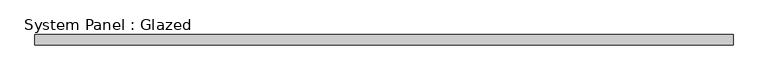
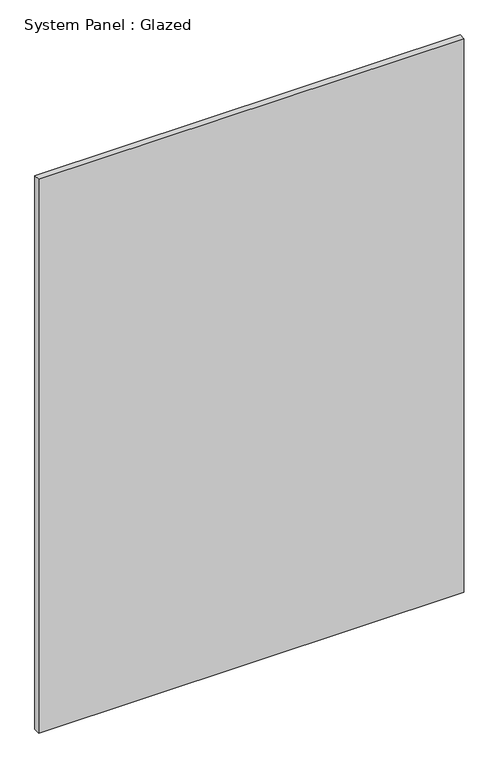
"""IFC4 building model written with IfcOpenShell, lengths in millimetres: plate geometry, System Panel : Glazed."""

from ifc_helpers import new_model, si_unit, origin, origin_with_axes, place, context, project, spatial, polyline, outline, extrude, source, transform, mapped, element, save


def system_panel_glazed_2d78c1f3(model_context):
    return source(origin(), model_context, "Body", "SweptSolid", [
        extrude(outline(polyline([(850.9, 19.05), (-850.9, 19.05), (-850.9, 44.45), (850.9, 44.45), (850.9, 19.05)])), origin_with_axes(), (0.0, 0.0, 1.0), 2343.15),
    ])


if __name__ == "__main__":
    model = new_model("IFC4")
    model_context = context("Model", 3, world=origin())
    ifc_project = project(units=[si_unit("LENGTHUNIT", "METRE", prefix="MILLI")], contexts=[model_context])
    site = spatial("IfcSite", under=ifc_project)
    building = spatial("IfcBuilding", under=site)
    placement = place(None, origin())
    system_panel_glazed_shape = system_panel_glazed_2d78c1f3(model_context)
    element("IfcPlate", 1, ObjectType="System Panel : Glazed", at=placement, inside=building, context=model_context, shape_type="MappedRepresentation", body=[
        mapped(system_panel_glazed_shape, transform((0.0, 0.0, 0.0), x_axis=(1.0, 0.0, 0.0), y_axis=(0.0, 1.0, 0.0), z_axis=(0.0, 0.0, 1.0))),
    ])
    save(model, "model.ifc")

# Revit data of these elements
# Type "System Panel : Glazed"
#   Construction Type Id = "GSP4R"
#   Analytic Construction = "1/8 in Pilkington single glazing"
#   Visual Light Transmittance = 0.9
#   Solar Heat Gain Coefficient = 0.86
#   Heat Transfer Coefficient (U) = 1.18115 BTU/(h·ft²·°F)
# Element 1 (IfcPlate, "System Panel : Glazed")
#   Materials on its faces: "Glass"
# Materials
#   "Glass": class "Glass", colour RGB 0 128 192, transparency 0.75, Description = "Soda Lime Glass", Cost = 0
